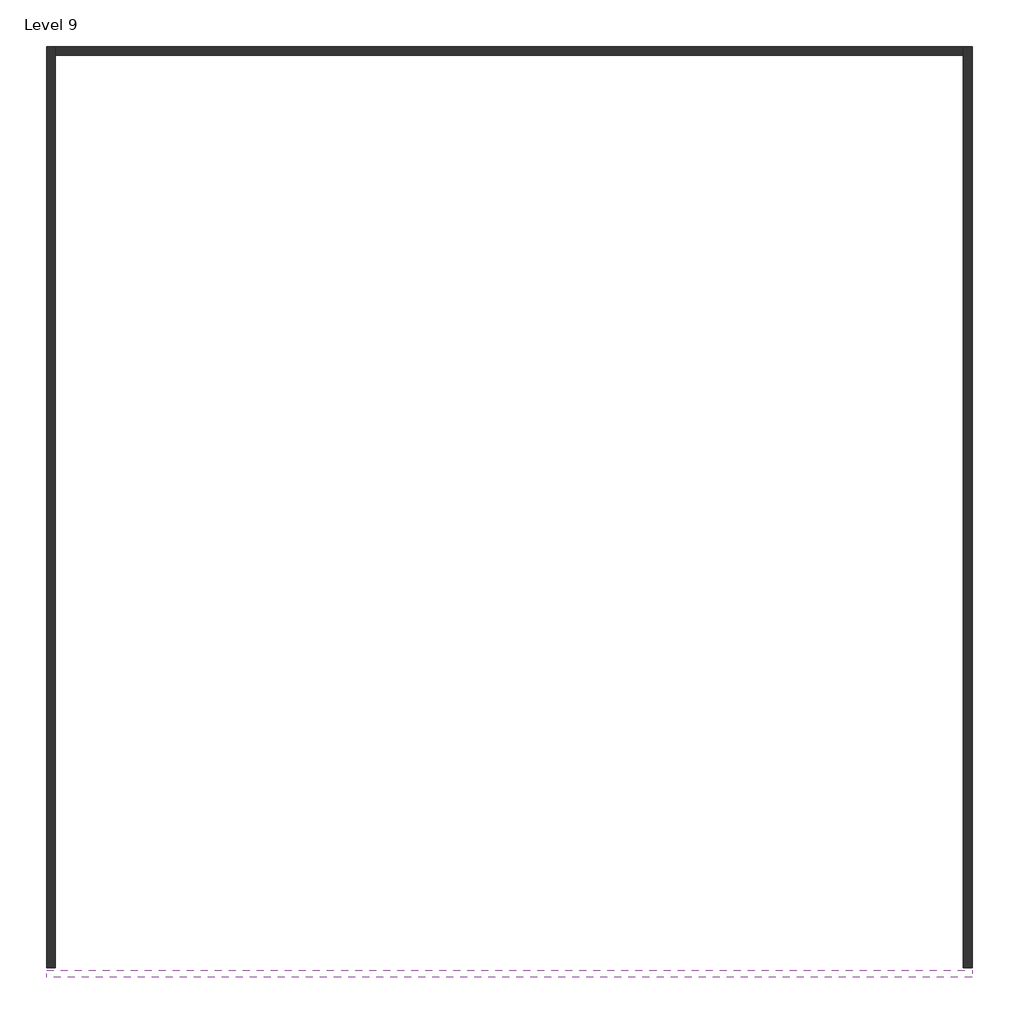
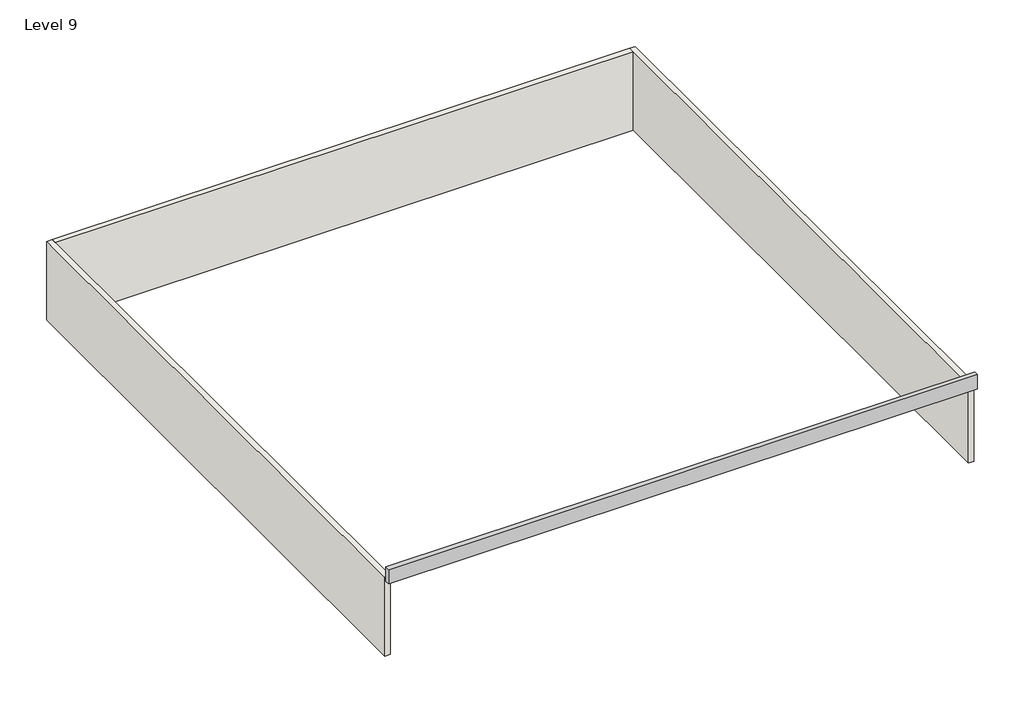
# One storey: 3 walls, 1 proxy.
"""IFC4 building model written with IfcOpenShell, lengths in millimetres."""

from ifc_helpers import new_model, si_unit, frame, origin, place, context, project, spatial, polyline, outline, extrude, faceted_brep, transform, mapped, element, save
from components import generic_models_7_generic_models_7_d0c4d58f

model = new_model("IFC4")

# Units and contexts
model_context = context("Model", 3, world=origin())
ifc_project = project(units=[si_unit("LENGTHUNIT", "METRE", prefix="MILLI")], contexts=[model_context])

# Site, building, storey
site = spatial("IfcSite", under=ifc_project)
building = spatial("IfcBuilding", under=site)
storey = spatial("IfcBuildingStorey", under=building, Name="Level 9", Elevation=13106.4)

# Proxy
placement = place(None, origin())
generic_models_7_generic_models_7_shape = generic_models_7_generic_models_7_d0c4d58f(model_context)
element("IfcBuildingElementProxy", 1, Name="Generic Models 7 : Generic Models 7", ObjectType="Generic Models 7 : Generic Models 7", at=placement, inside=storey, context=model_context, shape_type="MappedRepresentation", body=[
    mapped(generic_models_7_generic_models_7_shape, transform((0.0, 0.0, 0.0), x_axis=(1.0, 0.0, 0.0), y_axis=(0.0, 1.0, 0.0), z_axis=(0.0, 0.0, 1.0))),
])

# Walls
element("IfcWall", 2, ObjectType="outer wall", at=placement, inside=storey, context=model_context, shape_type="Brep", body=[
    faceted_brep([(-8731.5629849, -3682.5004242, 13106.4), (-8731.5629849, 17551.8995758, 13106.4), (-8731.5629849, 17755.0995758, 13106.4), (-8731.5629849, 17755.0995758, 16154.4), (-8731.5629849, 17551.8995758, 16154.4), (-8731.5629849, -3682.5004242, 16154.4), (-8934.7629849, -3682.5004242, 13106.4), (-8934.7629849, -3682.5004242, 16154.4), (-8934.7629849, 17755.0995758, 16154.4), (-8934.7629849, 17755.0995758, 13106.4)], [[[0, 1, 2, 3, 4, 5]], [[6, 7, 8, 9]], [[2, 1, 0, 6, 9]], [[0, 5, 7, 6]], [[5, 4, 3, 8, 7]], [[3, 2, 9, 8]]]),
])
element("IfcWall", 3, ObjectType="outer wall", at=placement, inside=storey, context=model_context, shape_type="Brep", body=[
    faceted_brep([(12604.4370151, -3682.5004242, 13106.4), (12604.4370151, 17755.0995758, 13106.4), (12604.4370151, 17755.0995758, 16154.4), (12604.4370151, -3682.5004242, 16154.4), (12401.2370151, -3682.5004242, 13106.4), (12401.2370151, -3682.5004242, 16154.4), (12401.2370151, 17551.8995758, 16154.4), (12401.2370151, 17755.0995758, 16154.4), (12401.2370151, 17755.0995758, 13106.4), (12401.2370151, 17551.8995758, 13106.4)], [[[0, 1, 2, 3]], [[4, 5, 6, 7, 8, 9]], [[1, 0, 4, 9, 8]], [[0, 3, 5, 4]], [[3, 2, 7, 6, 5]], [[2, 1, 8, 7]]]),
])
element("IfcWall", 4, ObjectType="outer wall", at=placement, inside=storey, context=model_context, shape_type="SweptSolid", body=[
    extrude(outline(polyline([(12401.2370151, 17551.8995758), (-8731.5629849, 17551.8995758), (-8731.5629849, 17755.0995758), (12401.2370151, 17755.0995758), (12401.2370151, 17551.8995758)])), frame((0.0, 0.0, 13106.4), z_axis=(0.0, 0.0, 1.0), x_axis=(1.0, 0.0, 0.0)), (0.0, 0.0, 1.0), 3048.0),
])

save(model, "model.ifc")

# Revit data of these elements
# Type "outer wall"
#   Assembly Code = "B2010"
#   Layers, outside or top first: 0' - 8" "Copper" (function 1)
# Element 1 (IfcBuildingElementProxy, "Generic Models 7 : Generic Models 7")
#   Phase Created = New Construction
# Elements 2, 3, 4 (IfcWall, "outer wall")
#   Top Offset = 0' - 0"
#   Base Offset = 0' - 0"
#   Unconnected Height = 10' - 0"
#   wall height = 10' - 0"
#   Phase Created = New Construction
#   Base Constraint = Level 9
#   Materials on its faces: "Copper"
# Materials
#   "Copper": class "Metal", colour RGB 0 0 0, transparency 0, Description = "Copper, matte finish", Cost = 0
